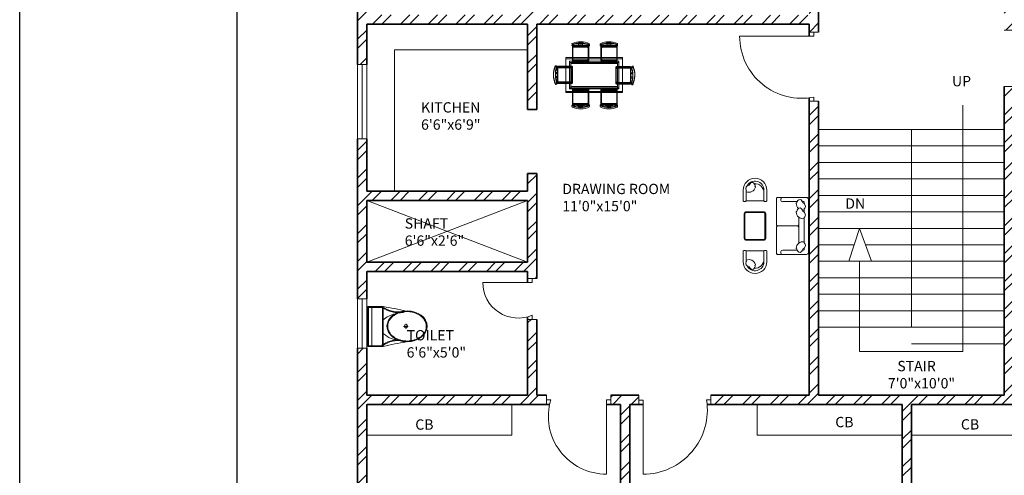
# Model space of a CAD drawing. Units: inches. Extents: x 2168 to 3056, y 1130 to 2629.
# Tile 2 of 42: x 2168 to 2645, y 1568 to 1789. Entities that reach past the tile are written whole.
import ezdxf

# ---------------------------------------------------------------- set-up
doc = ezdxf.new("R2010")
doc.units = ezdxf.units.IN
for name, color, linetype, lineweight in [('A-ANNO-DIMS', 2, 'Continuous', 18), ('A-ANNO-TEXT', 7, 'Continuous', 18), ('A-ANNO-TTLB', 7, 'Continuous', 25), ('A-AREA-IDEN', 7, 'Continuous', 18), ('A-DOOR', 21, 'Continuous', 18), ('A-FLOR-CASE', 71, 'Continuous', 18), ('A-FLOR-FIXT', 9, 'Continuous', 18), ('A-FLOR-OTLN', 7, 'Continuous', 18), ('A-FLOR-STRS', 71, 'Continuous', 18), ('A-FURN', 8, 'Continuous', 13), ('A-GLAZ', 201, 'Continuous', 18), ('A-WALL', 7, 'Continuous', 35)]:
    doc.layers.add(name, color=color, linetype=linetype, lineweight=lineweight)
doc.layers.add('A-WALL-PATT', color=143, linetype='Continuous', lineweight=13, true_color=0x7aafdf)
doc.styles.get("Standard").update_dxf_attribs({"font": 'arial.ttf'})
doc.dimstyles.get("Standard").update_dxf_attribs({"dimtxt": 0.18, "dimasz": 0.18, "dimexe": 0.18, "dimexo": 0.0625, "dimgap": 0.09, "dimtad": 0, "dimtih": 1, "dimtoh": 1, "dimdec": 4, "dimzin": 0, "dimdsep": 46, "dimtxsty": 'Standard', "dimcen": 0.09, "dimadec": 0, "dimazin": 0, "dimtfac": 1, "dimtdec": 4, "dimtofl": 0, "dimtmove": 0, "dimatfit": 3, "dimfxl": 1, "dimtolj": 1, "dimtzin": 0, "dimarcsym": 0})

# ---------------------------------------------------------------- blocks, each defined once
blk = doc.blocks.new('A$C31115884')
for p, q in [((258, 466), (258, 523)), ((283, 498), (223, 498)), ((0, 200), (0, 0)), ((520, 200), (0, 200)), ((10, 190), (10, 10)), ((510, 190), (10, 190)), ((510, 10), (510, 190)), ((520, 0), (520, 200)), ((510, 54), (0, 54)), ((10, 10), (510, 10)), ((0, 0), (520, 0))]:
    blk.add_line(p, q)
blk.add_circle((256, 496), 23.6)
for centre, radius, start, end in [((2778, -205), 2807, 165.4549, 171.7133), ((-295, 403), 365, 324.2091, 9.3499), ((-295, 403), 375, 324.2091, 9.3499), ((139, 406), 293, 315.8436, 2.6563), ((806, 403), 375, 179.2036, 215.7909), ((806, 403), 365, 170.6501, 215.7909), ((3237, 905), 2807, 188.2867, 194.5451), ((384, 406), 293, 190.2774, 224.1564)]:
    blk.add_arc(centre, radius, start, end)
blk.add_ellipse((256, 510), major_axis=(0, -261), ratio=0.772727)
blk.add_open_spline([(256, 259), (263, 259), (270, 260), (288, 262), (299, 265), (320, 273), (330, 278), (350, 291), (360, 299), (378, 316), (386, 326), (402, 347), (409, 358), (421, 383), (427, 395), (436, 422), (440, 436), (445, 465), (447, 480), (448, 509), (448, 524), (445, 553), (443, 568), (436, 596), (432, 610), (422, 636), (416, 649), (402, 672), (395, 683), (379, 703), (370, 712), (351, 728), (341, 735), (321, 746), (310, 751), (289, 757), (278, 759), (256, 761), (245, 761), (223, 757), (212, 754), (191, 746), (181, 741), (161, 728), (151, 720), (133, 703), (125, 693), (110, 672), (103, 660), (90, 636), (85, 623), (76, 596), (72, 582), (67, 553), (66, 538), (64, 509), (65, 494), (68, 465), (70, 450), (77, 422), (81, 408), (91, 382), (97, 370), (111, 346), (118, 335), (135, 316), (144, 307), (162, 291), (172, 284), (193, 273), (203, 269), (225, 262), (236, 260), (250, 259), (253, 259), (256, 259)], degree=3, knots=[0, 0, 0, 0, 0.110105, 0.110105, 0.285049, 0.285049, 0.459994, 0.459994, 0.634938, 0.634938, 0.809882, 0.809882, 0.984827, 0.984827, 1.159771, 1.159771, 1.334715, 1.334715, 1.50966, 1.50966, 1.684604, 1.684604, 1.859549, 1.859549, 2.034493, 2.034493, 2.209437, 2.209437, 2.384382, 2.384382, 2.559326, 2.559326, 2.73427, 2.73427, 2.909215, 2.909215, 3.084159, 3.084159, 3.259103, 3.259103, 3.434048, 3.434048, 3.608992, 3.608992, 3.783936, 3.783936, 3.958881, 3.958881, 4.133825, 4.133825, 4.30877, 4.30877, 4.483714, 4.483714, 4.658658, 4.658658, 4.833603, 4.833603, 5.008547, 5.008547, 5.183491, 5.183491, 5.358436, 5.358436, 5.53338, 5.53338, 5.708324, 5.708324, 5.883269, 5.883269, 6.058213, 6.058213, 6.233158, 6.233158, 6.283185, 6.283185, 6.283185, 6.283185])
blk = doc.blocks.new('A$C1352')
at = {"color": 0}
for points in [[(0.003, 0.053), (0.003, 0.553, -0.414214), (0.053, 0.603), (0.753, 0.603, -0.414214), (0.803, 0.553), (0.803, 0.053, -0.414214), (0.753, 0.003), (0.053, 0.003, -0.414214)], [(0.023, 0.053), (0.023, 0.553, -0.414214), (0.053, 0.583), (0.753, 0.583, -0.414214), (0.783, 0.553), (0.783, 0.053, -0.414214), (0.753, 0.023), (0.053, 0.023, -0.414214)]]:
    blk.add_lwpolyline(points, format="xyb", close=True, dxfattribs=at)
blk = doc.blocks.new('CHAIR-LOUNGE')
blk.add_line((10.04, 5.71), (10.04, 10.98))
at = {"ltscale": 0.03}
blk.add_lwpolyline([(10.04, 10.98, -0.369229), (11.42, 10.98), (11.42, 5.7, -1), (0, 5.72), (0, 10.99, -0.369229), (1.39, 10.99)], format="xyb", close=True, dxfattribs=at)
blk.add_lwpolyline([(9.55, 3.71, -0.785087), (1.38, 5.71), (1.39, 10.99)], format="xyb")
for centre, radius, start, end in [((5.71, 6.93), 4.33, 179.9461, 273.658), ((8.67, 3.43), 3.35, 67.0143, 164.2857), ((8.41, 5.02), 1.73, 272.9922, 34.1401), ((5.71, 5.71), 4.33, 358.8536, 359.9461), ((5.63, 4.23), 0.207, 150.6238, 293.7423), ((7.44, 3.63), 1.78, 166.6403, 249.4695), ((6.65, 3.91), 1.95, 274.9999, 341.3534)]:
    blk.add_arc(centre, radius, start, end)
blk = doc.blocks.new('TABLE-DINING')
for points in [[(0, 17.02), (27.45, 17.02), (27.45, 0.55), (0, 0.55)], [(0, 17.02), (27.45, 17.02), (27.45, 0.55), (0, 0.55)], [(0, 16.47), (27.45, 16.47), (27.45, 0), (0, 0)], [(0, 16.47), (27.45, 16.47), (27.45, 0), (0, 0)], [(1.83, 15.19), (25.62, 15.19), (25.62, 2.38), (1.83, 2.38)], [(1.83, 15.19), (25.62, 15.19), (25.62, 2.38), (1.83, 2.38)], [(1.83, 14.64), (25.62, 14.64), (25.62, 1.83), (1.83, 1.83)], [(1.83, 14.64), (25.62, 14.64), (25.62, 1.83), (1.83, 1.83)], [(2.38, 14.64), (25.07, 14.64), (25.07, 2.93), (2.38, 2.93)], [(2.38, 14.64), (25.07, 14.64), (25.07, 2.93), (2.38, 2.93)], [(2.38, 14.09), (25.07, 14.09), (25.07, 2.38), (2.38, 2.38)], [(2.38, 14.09), (25.07, 14.09), (25.07, 2.38), (2.38, 2.38)]]:
    blk.add_lwpolyline(points, close=True)
blk = doc.blocks.new('CUPBOARD-BEDROOM')
blk.add_lwpolyline([(0, 14.89), (70.36, 14.89), (70.36, 0), (0, 0)], close=True)
blk = doc.blocks.new('CHAIR-DINING-SIDE')
for points in [[(7.85, 2.38, 0.414214), (8.33, 2.86), (8.33, 9.24, 0.414214), (7.85, 9.73), (0.91, 9.73, 0.414214), (0.42, 9.24), (0.42, 2.86, 0.414214), (0.91, 2.38), (7.85, 2.38)], [(7.85, 2.38, 0.414214), (8.33, 2.86), (8.33, 9.24, 0.414214), (7.85, 9.73), (0.91, 9.73, 0.414214), (0.42, 9.24), (0.42, 2.86, 0.414214), (0.91, 2.38), (7.85, 2.38)], [(7.85, 1.83, 0.414214), (8.33, 2.31), (8.33, 8.69, 0.414214), (7.85, 9.18), (0.91, 9.18, 0.414214), (0.42, 8.69), (0.42, 2.31, 0.414214), (0.91, 1.83), (7.85, 1.83)], [(7.85, 1.83, 0.414214), (8.33, 2.31), (8.33, 8.69, 0.414214), (7.85, 9.18), (0.91, 9.18, 0.414214), (0.42, 8.69), (0.42, 2.31, 0.414214), (0.91, 1.83), (7.85, 1.83)], [(8.06, 2.08, -0.175809), (0.59, 2.13, 0.578392), (0.02, 1.51, 0.214524), (8.46, 1.4, 0.552014), (8.06, 2.08, -0.065079)], [(8.06, 2.08, -0.175809), (0.59, 2.13, 0.578392), (0.02, 1.51, 0.214524), (8.46, 1.4, 0.552014), (8.06, 2.08, -0.065079)], [(8.06, 1.53, -0.175809), (0.59, 1.58, 0.578392), (0.02, 0.96, 0.214524), (8.46, 0.85, 0.552014), (8.06, 1.53, -0.065079)], [(8.06, 1.53, -0.175809), (0.59, 1.58, 0.578392), (0.02, 0.96, 0.214524), (8.46, 0.85, 0.552014), (8.06, 1.53, -0.065079)], [(3.34, 2.38), (3.34, 1.5, -0.064759)], [(3.34, 2.38), (3.34, 1.5, -0.064759)], [(3.34, 1.83), (3.34, 0.95, -0.064759)], [(3.34, 1.83), (3.34, 0.95, -0.064759)]]:
    blk.add_lwpolyline(points, format="xyb")
for points in [[(7.84, 2.6), (1.13, 2.6, -0.414214), (0.64, 3.08), (0.64, 9.02, -0.414214), (1.13, 9.51), (7.84, 9.51, -0.512069), (8.11, 9.02), (8.11, 3.08, -0.512069)], [(7.84, 2.6), (1.13, 2.6, -0.414214), (0.64, 3.08), (0.64, 9.02, -0.414214), (1.13, 9.51), (7.84, 9.51, -0.512069), (8.11, 9.02), (8.11, 3.08, -0.512069)], [(7.84, 2.05), (1.13, 2.05, -0.414214), (0.64, 2.53), (0.64, 8.48, -0.414214), (1.13, 8.96), (7.84, 8.96, -0.512069), (8.11, 8.48), (8.11, 2.53, -0.512069)], [(7.84, 2.05), (1.13, 2.05, -0.414214), (0.64, 2.53), (0.64, 8.48, -0.414214), (1.13, 8.96), (7.84, 8.96, -0.512069), (8.11, 8.48), (8.11, 2.53, -0.512069)]]:
    blk.add_lwpolyline(points, format="xyb", close=True)
for points in [[(5.29, 1.48), (5.29, 2.38)], [(5.29, 1.48), (5.29, 2.38)], [(5.29, 0.93), (5.29, 1.83)], [(5.29, 0.93), (5.29, 1.83)]]:
    blk.add_lwpolyline(points)
blk = doc.blocks.new('CHAIR-DINING-END')
for points in [[(1.58, 1.14, -0.578392), (0.96, 0.57, -0.214524), (0.85, 9.01, -0.552014), (1.53, 8.61, 0.175809), (1.58, 1.14)], [(1.58, 1.14, -0.578392), (0.96, 0.57, -0.214524), (0.85, 9.01, -0.552014), (1.53, 8.61, 0.175809), (1.58, 1.14)], [(1.58, 0.59, -0.578392), (0.96, 0.02, -0.214524), (0.85, 8.46, -0.552014), (1.53, 8.06, 0.175809), (1.58, 0.59)], [(1.58, 0.59, -0.578392), (0.96, 0.02, -0.214524), (0.85, 8.46, -0.552014), (1.53, 8.06, 0.175809), (1.58, 0.59)], [(1.83, 8.39, -0.414214), (2.31, 8.88), (8.69, 8.88, -0.414214), (9.18, 8.39), (9.18, 1.45, -0.414214), (8.69, 0.97), (2.31, 0.97, -0.414214), (1.83, 1.45), (1.83, 8.39)], [(1.83, 8.39, -0.414214), (2.31, 8.88), (8.69, 8.88, -0.414214), (9.18, 8.39), (9.18, 1.45, -0.414214), (8.69, 0.97), (2.31, 0.97, -0.414214), (1.83, 1.45), (1.83, 8.39)], [(1.83, 7.85, -0.414214), (2.31, 8.33), (8.69, 8.33, -0.414214), (9.18, 7.85), (9.18, 0.91, -0.414214), (8.69, 0.42), (2.31, 0.42, -0.414214), (1.83, 0.91), (1.83, 7.85)], [(1.83, 7.85, -0.414214), (2.31, 8.33), (8.69, 8.33, -0.414214), (9.18, 7.85), (9.18, 0.91, -0.414214), (8.69, 0.42), (2.31, 0.42, -0.414214), (1.83, 0.91), (1.83, 7.85)], [(1.83, 3.89), (0.95, 3.89, 0.064759)], [(1.83, 3.89), (0.95, 3.89, 0.064759)], [(1.83, 3.34), (0.95, 3.34, 0.064759)], [(1.83, 3.34), (0.95, 3.34, 0.064759)]]:
    blk.add_lwpolyline(points, format="xyb")
for points in [[(0.93, 5.84), (1.83, 5.84)], [(0.93, 5.83), (1.83, 5.83)], [(0.93, 5.29), (1.83, 5.29)], [(0.93, 5.29), (1.83, 5.29)]]:
    blk.add_lwpolyline(points)
for points in [[(2.05, 8.39), (2.05, 1.67, 0.414214), (2.53, 1.19), (8.48, 1.19, 0.414214), (8.96, 1.67), (8.96, 8.39, 0.512069), (8.48, 8.66), (2.53, 8.66, 0.512069)], [(2.05, 8.39), (2.05, 1.67, 0.414214), (2.53, 1.19), (8.48, 1.19, 0.414214), (8.96, 1.67), (8.96, 8.39, 0.512069), (8.48, 8.66), (2.53, 8.66, 0.512069)], [(2.05, 7.84), (2.05, 1.12, 0.414214), (2.53, 0.64), (8.48, 0.64, 0.414214), (8.96, 1.12), (8.96, 7.84, 0.512069), (8.48, 8.11), (2.53, 8.11, 0.512069)], [(2.05, 7.84), (2.05, 1.12, 0.414214), (2.53, 0.64), (8.48, 0.64, 0.414214), (8.96, 1.12), (8.96, 7.84, 0.512069), (8.48, 8.11), (2.53, 8.11, 0.512069)]]:
    blk.add_lwpolyline(points, format="xyb", close=True)
blk = doc.blocks.new('WIN-24-OPPOSED-JAMBS')
for p, q in [((0, 4.5), (0, 0)), ((0, 4.5), (24, 4.5)), ((0, 0), (0, 2.25)), ((0, 2.25), (24, 2.25)), ((24, 2.25), (24, 4.5)), ((24, 4.5), (24, 0)), ((0, 0), (24, 0))]:
    blk.add_line(p, q)
blk = doc.blocks.new('WIN-36')
for p, q in [((2.25, 36), (0, 36)), ((0, 36), (4.5, 36)), ((0, 36), (0, 0)), ((2.25, 0), (2.25, 36)), ((4.5, 36), (4.5, 0)), ((0, 0), (4.5, 0)), ((4.5, 0), (2.25, 0))]:
    blk.add_line(p, q)
blk = doc.blocks.new('*D41')
at = {"layer": 'A-ANNO-DIMS', "color": 0, "lineweight": -2, "transparency": 16777216}
for p, q in [((2331.73, 2478.39), (2273.32, 2478.39)), ((2273.5, 2478.21), (2273.5, 1928.07)), ((2273.5, 1377.57), (2273.5, 1927.71)), ((2331.73, 1377.39), (2273.32, 1377.39))]:
    blk.add_line(p, q, dxfattribs=at)
at = {"layer": 'A-ANNO-DIMS', "color": 0, "transparency": 16777216}
for points in [[(2273.47, 2478.21), (2273.53, 2478.21), (2273.5, 2478.39)], [(2273.47, 1377.57), (2273.53, 1377.57), (2273.5, 1377.39)]]:
    blk.add_solid(points, dxfattribs=at)
at = {"layer": 'Defpoints', "color": 0, "transparency": 16777216}
for p in [(2273.5, 2478.39), (2331.8, 2478.39), (2331.8, 1377.39)]:
    blk.add_point(p, dxfattribs=at)
at = {"layer": 'A-ANNO-DIMS', "color": 0, "transparency": 16777216, "insert": (2273.5, 1927.89), "char_height": 0.18, "attachment_point": 5}
blk.add_mtext('\\A1;1101', dxfattribs=at)

msp = doc.modelspace()

# ---------------------------------------------------------------- hatches: boundary and pattern name
at = {"layer": 'A-WALL-PATT'}
h = msp.add_hatch(dxfattribs=at)
h.set_pattern_fill('ANSI32', color=256)
h.paths.add_polyline_path([(2463.8, 2409.39), (2467.39, 2409.39), (2467.39, 2413.89), (2454.77, 2413.89), (2454.77, 2411.64), (2454.77, 2409.39), (2459.3, 2409.39), (2459.3, 2265.39), (2455.64, 2265.39), (2455.64, 2260.89), (2467.35, 2260.89), (2467.35, 2263.14), (2467.35, 2265.39), (2463.8, 2265.39)])
h.paths.add_polyline_path([(2431.6, 2413.89), (2409.65, 2413.89), (2409.65, 2409.39), (2431.6, 2409.39), (2431.6, 2411.64)])
h.paths.add_polyline_path([(2349.65, 2413.89), (2331.8, 2413.89), (2331.8, 2362.67), (2336.3, 2362.67), (2336.3, 2409.39), (2349.65, 2409.39), (2349.65, 2411.64)])
h.paths.add_polyline_path([(2634.15, 2411.64), (2634.15, 2413.89), (2562.29, 2413.89), (2562.29, 2409.39), (2595.8, 2409.39), (2595.8, 2280.31), (2595.83, 2280.31), (2595.83, 2265.39), (2499.91, 2265.39), (2499.91, 2260.89), (2550.8, 2260.89), (2550.8, 2117.31), (2555.3, 2117.31), (2555.3, 2168.08), (2571.93, 2168.08), (2571.93, 2176.89), (2559.8, 2176.89), (2559.8, 2256.39), (2640.8, 2256.39), (2640.8, 2176.89), (2626.43, 2176.89), (2626.43, 2168.08), (2645.3, 2168.08), (2645.3, 2116.64), (2649.8, 2116.64), (2649.8, 2260.89), (2691.25, 2260.89), (2691.25, 2263.14), (2691.25, 2265.39), (2670.65, 2265.39), (2670.65, 2265.36), (2600.3, 2265.36), (2600.3, 2280.26), (2600.3, 2409.39), (2634.15, 2409.39)])
h.paths.add_polyline_path([(2600.3, 2473.89), (2612.84, 2473.89), (2612.84, 2478.39), (2572.64, 2478.39), (2572.64, 2473.89), (2595.8, 2473.89), (2595.8, 2413.89), (2600.3, 2413.89)])
h.paths.add_polyline_path([(2535.8, 2473.89), (2548.64, 2473.89), (2548.64, 2478.39), (2531.4, 2478.39), (2531.4, 2413.89), (2521.6, 2413.89), (2521.6, 2409.39), (2539.24, 2409.39), (2539.24, 2411.64), (2539.24, 2413.89), (2535.8, 2413.89)])
h.paths.add_polyline_path([(2664.8, 2478.39), (2636.84, 2478.39), (2636.84, 2473.89), (2660.3, 2473.89), (2660.3, 2413.89), (2656.17, 2413.89), (2656.17, 2409.39), (2671.68, 2409.39), (2671.68, 2411.64), (2671.68, 2413.89), (2664.8, 2413.89)])
h.paths.add_polyline_path([(2705.94, 2413.89), (2695.68, 2413.89), (2695.68, 2409.39), (2705.94, 2409.39)])
h.paths.add_polyline_path([(2741.35, 2413.89), (2728.73, 2413.89), (2728.73, 2411.64), (2728.73, 2409.39), (2732.3, 2409.39), (2732.3, 2265.39), (2725.73, 2265.39), (2725.73, 2260.89), (2740.92, 2260.89), (2740.92, 2263.14), (2740.92, 2265.39), (2736.8, 2265.39), (2736.8, 2409.39), (2741.35, 2409.39)])
h.paths.add_polyline_path([(2785.65, 2413.89), (2764.55, 2413.89), (2764.49, 2409.39), (2785.65, 2409.39), (2785.65, 2411.64)])
h.paths.add_polyline_path([(2864.3, 2413.89), (2845.65, 2413.89), (2845.65, 2409.39), (2859.8, 2409.39), (2859.8, 2368.43), (2864.3, 2368.43)])
h.paths.add_polyline_path([(2864.3, 2308.43), (2862.05, 2308.43), (2859.8, 2308.43), (2859.8, 2265.39), (2774.48, 2265.39), (2774.48, 2263.14), (2774.48, 2260.89), (2781.8, 2260.89), (2781.8, 2226.65), (2786.3, 2226.65), (2786.3, 2260.89), (2859.8, 2260.89), (2859.8, 2241.35), (2864.3, 2241.35)])
h.paths.add_polyline_path([(2864.3, 2217.35), (2862.05, 2217.35), (2859.8, 2217.35), (2859.8, 2200.89), (2786.3, 2200.89), (2786.3, 2205.93), (2784.05, 2205.93), (2781.8, 2205.93), (2781.8, 2150.97), (2786.3, 2150.97), (2786.3, 2161.89), (2859.8, 2161.89), (2859.8, 2144.42), (2864.3, 2144.42)])
h.paths.add_polyline_path([(2859.8, 2196.39), (2859.8, 2166.39), (2786.3, 2166.39), (2786.3, 2196.39)], flags=16)
h.paths.add_polyline_path([(2864.3, 2108.42), (2862.05, 2108.42), (2859.8, 2108.42), (2859.8, 2080.89), (2786.3, 2080.89), (2786.3, 2111.99), (2781.8, 2111.99), (2781.8, 2080.89), (2649.8, 2080.89), (2649.8, 2086.04), (2647.55, 2086.04), (2645.3, 2086.04), (2645.3, 2071.74), (2649.8, 2071.74), (2649.8, 2076.39), (2781.8, 2076.39), (2781.8, 2041.79), (2786.3, 2041.79), (2786.3, 2076.39), (2859.8, 2076.39), (2859.8, 2058.58), (2864.3, 2058.58)])
h.paths.add_polyline_path([(2864.3, 2022.58), (2859.8, 2022.58), (2859.8, 1992.39), (2786.3, 1992.39), (2786.3, 1999.57), (2781.8, 1999.57), (2781.8, 1848.09), (2784.05, 1848.09), (2786.3, 1848.09), (2786.3, 1851.39), (2859.8, 1851.39), (2859.8, 1838.26), (2864.3, 1838.26)], flags=17)
h.paths.add_polyline_path([(2859.8, 1987.89), (2859.8, 1855.89), (2786.3, 1855.89), (2786.3, 1987.89)], flags=16)
h.paths.add_polyline_path([(2823.05, 1987.89), (2841.42, 1921.89), (2823.05, 1855.89)], flags=0)
h.paths.add_polyline_path([(2864.3, 1814.26), (2859.8, 1814.26), (2859.8, 1791.39), (2786.3, 1791.39), (2786.3, 1825.66), (2784.05, 1825.66), (2781.8, 1825.66), (2781.8, 1791.39), (2720.15, 1791.39), (2720.15, 1791.27), (2649.8, 1791.27), (2649.8, 1806.16), (2649.8, 2038.98), (2647.55, 2038.98), (2645.3, 2038.98), (2645.3, 1783.93), (2649.8, 1783.93), (2649.8, 1786.89), (2781.8, 1786.89), (2781.8, 1746.79), (2786.3, 1746.79), (2786.3, 1786.89), (2859.8, 1786.89), (2859.8, 1770.08), (2864.3, 1770.08)])
h.paths.add_polyline_path([(2864.3, 1734.08), (2862.05, 1734.08), (2859.8, 1734.08), (2859.8, 1705.89), (2786.3, 1705.89), (2786.3, 1714.17), (2781.8, 1714.17), (2781.8, 1660.53), (2786.3, 1660.53), (2786.3, 1666.89), (2859.8, 1666.89), (2859.8, 1648.34), (2864.3, 1648.34)])
h.paths.add_polyline_path([(2786.3, 1701.39), (2859.8, 1701.39), (2859.8, 1671.39), (2786.3, 1671.39)], flags=16)
h.paths.add_polyline_path([(2649.8, 1756.58), (2647.55, 1756.58), (2645.3, 1756.58), (2645.3, 1606.89), (2555.3, 1606.89), (2555.3, 1749.51), (2553.05, 1749.51), (2550.8, 1749.51), (2550.8, 1606.89), (2503.01, 1606.89), (2503.01, 1604.64), (2503.01, 1602.39), (2595.8, 1602.39), (2595.85, 1602.39), (2595.85, 1587.5), (2595.8, 1458.39), (2561.5, 1458.39), (2561.5, 1456.14), (2561.5, 1453.89), (2595.8, 1453.89), (2595.8, 1381.89), (2573.44, 1381.89), (2573.44, 1377.39), (2613.01, 1377.39), (2613.01, 1379.64), (2613.01, 1381.89), (2600.3, 1381.89), (2600.3, 1453.89), (2634.33, 1453.89), (2634.33, 1458.39), (2600.3, 1458.39), (2600.3, 1602.39), (2670.65, 1602.39), (2694.09, 1602.39), (2694.09, 1606.89), (2649.8, 1606.89)])
h.paths.add_polyline_path([(2736.8, 1602.39), (2741.56, 1602.39), (2741.56, 1606.89), (2726.2, 1606.89), (2726.2, 1604.64), (2726.2, 1602.39), (2732.3, 1602.39), (2732.3, 1458.39), (2727.9, 1458.39), (2727.9, 1453.89), (2740.82, 1453.89), (2740.82, 1456.14), (2740.82, 1458.39), (2736.8, 1458.39)])
h.paths.add_polyline_path([(2859.8, 1606.89), (2786.3, 1606.89), (2786.3, 1637.33), (2784.05, 1637.33), (2781.8, 1637.33), (2781.8, 1606.89), (2775.61, 1606.89), (2775.61, 1602.39), (2859.8, 1602.39)])
h.paths.add_polyline_path([(2864.3, 1624.34), (2862.05, 1624.34), (2859.8, 1624.34), (2859.8, 1570.39), (2864.3, 1570.39)])
h.paths.add_polyline_path([(2864.3, 1510.39), (2862.05, 1510.39), (2859.8, 1510.39), (2859.8, 1458.39), (2846.73, 1458.39), (2846.73, 1456.14), (2846.73, 1453.89), (2864.3, 1453.89)])
h.paths.add_polyline_path([(2786.73, 1458.39), (2765.44, 1458.39), (2765.44, 1453.89), (2786.73, 1453.89)])
h.paths.add_polyline_path([(2706, 1458.39), (2695.36, 1458.39), (2695.36, 1453.89), (2706, 1453.89), (2706, 1456.14)])
h.paths.add_polyline_path([(2671.36, 1456.14), (2671.36, 1458.39), (2655.99, 1458.39), (2655.99, 1456.14), (2655.99, 1453.89), (2660.3, 1453.89), (2660.3, 1381.89), (2637.01, 1381.89), (2637.01, 1377.39), (2664.8, 1377.39), (2664.8, 1453.89), (2671.36, 1453.89)], flags=17)
h.paths.add_polyline_path([(2539.83, 1458.39), (2520.24, 1458.39), (2520.24, 1453.89), (2531.3, 1453.89), (2531.3, 1377.39), (2546.45, 1377.39), (2546.45, 1379.64), (2546.45, 1381.89), (2535.8, 1381.89), (2535.8, 1453.89), (2539.83, 1453.89)], flags=17)
h.paths.add_polyline_path([(2496.24, 1458.39), (2489.13, 1458.39), (2489.13, 1453.89), (2496.24, 1453.89), (2496.24, 1456.14)])
h.paths.add_polyline_path([(2467.43, 1456.14), (2467.43, 1458.39), (2463.8, 1458.39), (2463.8, 1602.39), (2468.24, 1602.39), (2468.24, 1605.7), (2468.24, 1606.89), (2454.6, 1606.89), (2454.6, 1602.39), (2459.3, 1602.39), (2459.3, 1458.39), (2454.24, 1458.39), (2454.24, 1453.89), (2467.43, 1453.89)])
h.paths.add_polyline_path([(2431.6, 1456.14), (2431.6, 1458.39), (2411.39, 1458.39), (2411.39, 1453.89), (2431.6, 1453.89)])
h.paths.add_polyline_path([(2351.39, 1458.39), (2336.3, 1458.39), (2336.3, 1490.69), (2334.05, 1490.69), (2331.8, 1490.69), (2331.8, 1453.89), (2351.39, 1453.89), (2351.39, 1456.14)])
h.paths.add_polyline_path([(2336.3, 1629.7), (2331.8, 1629.7), (2331.8, 1552.32), (2336.3, 1552.32), (2336.3, 1602.39), (2406.65, 1602.39), (2423.47, 1602.39), (2423.47, 1606.89), (2418.8, 1606.89), (2418.8, 1643.68), (2416.55, 1643.68), (2414.3, 1643.68), (2414.3, 1606.89), (2336.3, 1606.89)])
h.paths.add_polyline_path([(2418.8, 1714.38), (2414.3, 1714.38), (2414.3, 1705.89), (2336.3, 1705.89), (2336.3, 1731.32), (2334.05, 1731.32), (2331.8, 1731.32), (2331.8, 1653.7), (2334.05, 1653.7), (2336.3, 1653.7), (2336.3, 1666.89), (2414.3, 1666.89), (2414.3, 1663.59), (2418.8, 1663.59)])
h.paths.add_polyline_path([(2336.3, 1701.39), (2414.3, 1701.39), (2414.3, 1671.39), (2336.3, 1671.39)], flags=16)
h.paths.add_polyline_path([(2555.3, 2040.06), (2550.8, 2040.06), (2550.8, 1791.39), (2550.56, 1791.2), (2480.2, 1791.2), (2418.8, 1791.39), (2418.8, 1825.45), (2416.55, 1825.45), (2414.3, 1825.45), (2414.3, 1791.39), (2336.3, 1791.39), (2336.3, 1806.41), (2331.8, 1806.41), (2331.8, 1767.32), (2336.3, 1767.32), (2336.3, 1786.89), (2414.3, 1786.89), (2414.3, 1745.46), (2418.8, 1745.46), (2418.8, 1786.89), (2550.8, 1786.89), (2550.8, 1783.01), (2555.3, 1783.01)])
h.paths.add_polyline_path([(2418.8, 1923.39), (2423.21, 1923.39), (2423.21, 1925.64), (2423.21, 1927.89), (2418.8, 1927.89), (2418.8, 2000.05), (2414.3, 2000.05), (2414.3, 1992.39), (2336.3, 1992.39), (2336.3, 1987.89), (2414.3, 1987.89), (2414.3, 1855.89), (2336.3, 1855.89), (2336.3, 1851.39), (2414.3, 1851.39), (2414.3, 1846.76), (2418.8, 1846.76)], flags=17)
h.paths.add_polyline_path([(2336.3, 2019.29), (2334.05, 2019.29), (2331.8, 2019.29), (2331.8, 1830.41), (2336.3, 1830.41)], flags=17)
h.paths.add_polyline_path([(2550.8, 1927.89), (2453.54, 1927.89), (2453.54, 1925.64), (2453.54, 1923.39), (2550.8, 1923.39)], flags=17)
h.paths.add_polyline_path([(2744.99, 1927.89), (2649.8, 1927.89), (2649.8, 1923.39), (2744.99, 1923.39), (2744.99, 1925.64)], flags=17)
h.paths.add_polyline_path([(2555.3, 2086.46), (2553.05, 2086.46), (2550.8, 2086.46), (2550.8, 2080.89), (2418.8, 2080.89), (2336.3, 2080.89), (2336.3, 2115.4), (2334.05, 2115.4), (2331.8, 2115.4), (2331.8, 2055.29), (2336.3, 2055.29), (2336.3, 2076.39), (2550.8, 2076.39), (2550.8, 2071.54), (2555.3, 2071.54)])
h.paths.add_polyline_path([(2418.8, 2121.39), (2414.3, 2121.39), (2414.3, 2080.89), (2418.8, 2080.89)])
h.paths.add_polyline_path([(2418.8, 2076.39), (2414.3, 2076.39), (2414.3, 2035.12), (2418.8, 2035.12)])
h.paths.add_polyline_path([(2422.87, 2263.14), (2422.87, 2265.39), (2406.65, 2265.39), (2406.65, 2265.36), (2336.3, 2265.36), (2336.3, 2280.25), (2336.3, 2302.67), (2334.05, 2302.67), (2331.8, 2302.67), (2331.8, 2246.85), (2336.3, 2246.85), (2336.3, 2260.89), (2414.3, 2260.89), (2414.3, 2224), (2418.8, 2224), (2418.8, 2260.89), (2422.87, 2260.89)])
h.paths.add_polyline_path([(2418.8, 2204.78), (2416.55, 2204.78), (2414.3, 2204.78), (2414.3, 2200.89), (2336.3, 2200.89), (2336.3, 2220.85), (2331.8, 2220.85), (2331.8, 2151.4), (2336.3, 2151.4), (2336.3, 2161.89), (2414.3, 2161.89), (2414.3, 2153.73), (2418.8, 2153.73)])
h.paths.add_polyline_path([(2414.3, 2196.39), (2414.3, 2166.39), (2336.3, 2166.39), (2336.3, 2196.39)], flags=16)
h.paths.add_polyline_path([(2375.3, 2181.39), (2336.3, 2166.39), (2336.3, 2196.39)], flags=0)
h.paths.add_polyline_path([(2809.6, 2172.34), (2838.8, 2172.34), (2838.8, 2191), (2809.6, 2191)], flags=8)
h.paths.add_polyline_path([(2849.75, 1919.59), (2849.75, 1952.67), (2831.09, 1952.67), (2831.09, 1919.59)], flags=8)
h.paths.add_polyline_path([(2808.87, 1901.97), (2808.87, 1937.85), (2790.15, 1937.85), (2790.15, 1901.97)], flags=8)
h.paths.add_polyline_path([(2806.28, 1671.9), (2835.49, 1671.9), (2835.49, 1690.55), (2806.28, 1690.55)], flags=8)
h.paths.add_polyline_path([(2353.19, 1676.55), (2382.39, 1676.55), (2382.39, 1695.21), (2353.19, 1695.21)], flags=8)
h.paths.add_polyline_path([(2360.08, 1832.31), (2389.24, 1832.31), (2389.24, 1850.97), (2360.08, 1850.97)], flags=25)
h.paths.add_polyline_path([(2354.82, 2167.82), (2384.03, 2167.82), (2384.03, 2186.48), (2354.82, 2186.48)], flags=8)

# ---------------------------------------------------------------- linework, layer by layer
at = {"layer": 'A-ANNO-TTLB'}
msp.add_lwpolyline([(2168.16, 2629.19), (3055.63, 2629.19), (3055.63, 1130.19), (2168.16, 1130.19)], close=True, dxfattribs=at)
at = {"layer": 'A-DOOR'}
for p, q in [((2553.05, 1781.01), (2517.05, 1781.01)), ((2550.8, 1783.01), (2555.3, 1783.01)), ((2555.3, 1783.01), (2553.05, 1783.01)), ((2553.05, 1783.01), (2553.05, 1781.01)), ((2645.3, 1783.93), (2649.8, 1783.93)), ((2645.3, 1756.58), (2649.8, 1756.58)), ((2553.05, 1749.51), (2553.05, 1751.51)), ((2550.8, 1749.51), (2555.3, 1749.51)), ((2555.3, 1749.51), (2553.05, 1749.51)), ((2416.55, 1661.59), (2392.55, 1661.59)), ((2414.3, 1663.59), (2418.8, 1663.59)), ((2418.8, 1663.59), (2416.55, 1663.59)), ((2416.55, 1663.59), (2416.55, 1661.59)), ((2414.3, 1643.68), (2418.8, 1643.68)), ((2416.55, 1643.68), (2416.55, 1645.68)), ((2418.8, 1643.68), (2416.55, 1643.68)), ((2423.47, 1602.39), (2423.47, 1606.89)), ((2423.47, 1606.89), (2423.47, 1604.64)), ((2423.47, 1604.64), (2425.47, 1604.64)), ((2454.6, 1604.64), (2452.6, 1604.64)), ((2452.6, 1604.64), (2452.6, 1568.64)), ((2454.6, 1606.89), (2454.6, 1602.39)), ((2454.6, 1602.39), (2454.6, 1604.64)), ((2468.24, 1605.7), (2468.24, 1606.89)), ((2468.24, 1606.89), (2468.24, 1604.57)), ((2468.24, 1602.39), (2468.24, 1605.7)), ((2468.24, 1604.57), (2470.24, 1604.57)), ((2470.24, 1604.57), (2470.24, 1568.57)), ((2503.01, 1604.64), (2501.01, 1604.64)), ((2503.01, 1602.39), (2503.01, 1606.89)), ((2503.01, 1606.89), (2503.01, 1604.64))]:
    msp.add_line(p, q, dxfattribs=at)
for centre, radius, start, end in [((2547.13, 1781.01), 30.09, 180, 281.3384), ((2409.82, 1661.59), 17.27, 180, 292.9159), ((2452.44, 1596.74), 28.1, 163.6836, 270.3208), ((2470.24, 1599.73), 31.15, 270, 9.0691)]:
    msp.add_arc(centre, radius, start, end, dxfattribs=at)
at = {"layer": 'A-FLOR-CASE'}
for p, q in [((2414.3, 1774.45), (2349.78, 1774.45)), ((2349.78, 1774.45), (2349.78, 1705.89))]:
    msp.add_line(p, q, dxfattribs=at)
at = {"layer": 'A-FLOR-OTLN'}
for p, q in [((2336.3, 1671.39), (2414.3, 1701.39)), ((2336.3, 1701.39), (2414.3, 1671.39)), ((2414.3, 1701.39), (2414.3, 1701.39)), ((2336.3, 1671.39), (2336.3, 1671.39))]:
    msp.add_line(p, q, dxfattribs=at)
at = {"layer": 'A-FLOR-STRS'}
for p, q in [((2625.12, 1747.61), (2625.12, 1628.15)), ((2555.3, 1735.84), (2645.3, 1735.84)), ((2600.3, 1639.84), (2600.3, 1735.84)), ((2555.3, 1727.84), (2645.3, 1727.84)), ((2555.3, 1719.84), (2645.3, 1719.84)), ((2555.3, 1711.84), (2645.3, 1711.84)), ((2555.3, 1703.84), (2645.3, 1703.84)), ((2555.3, 1695.84), (2645.3, 1695.84)), ((2555.3, 1687.84), (2645.3, 1687.84)), ((2575.16, 1687.84), (2569.97, 1671.84)), ((2580.99, 1671.84), (2575.16, 1687.84)), ((2555.3, 1679.84), (2572.56, 1679.84)), ((2578.08, 1679.84), (2645.3, 1679.84)), ((2555.3, 1671.84), (2645.3, 1671.84)), ((2569.97, 1671.84), (2580.99, 1671.84)), ((2575.16, 1628.15), (2575.16, 1671.84)), ((2555.3, 1663.84), (2645.3, 1663.84)), ((2555.3, 1655.84), (2645.3, 1655.84)), ((2555.3, 1647.84), (2645.3, 1647.84)), ((2555.3, 1639.84), (2645.3, 1639.84)), ((2645.3, 1639.84), (2600.3, 1639.84)), ((2645.3, 1631.84), (2600.3, 1631.84)), ((2625.12, 1628.15), (2575.16, 1628.15))]:
    msp.add_line(p, q, dxfattribs=at)
at = {"layer": 'A-FURN'}
for p, q in [((2544.89, 1700.78), (2537.97, 1700.78)), ((2547.52, 1700.78), (2548, 1700.78)), ((2548.35, 1700.43), (2548.35, 1699.79)), ((2548.35, 1695.64), (2548.35, 1697.29)), ((2548.35, 1696.27), (2548.35, 1695.64)), ((2548.35, 1680.72), (2548.35, 1693.14)), ((2537.97, 1677.24), (2544.89, 1677.24)), ((2547.52, 1677.24), (2548, 1677.24)), ((2548.35, 1677.59), (2548.35, 1678.23))]:
    msp.add_line(p, q, dxfattribs=at)
for points in [[(2450.01, 1776.78, -0.578392), (2449.44, 1777.4, -0.214524), (2457.88, 1777.51, -0.552014), (2457.48, 1776.83, 0.175809), (2450.01, 1776.78)], [(2450.01, 1776.78, -0.578392), (2449.44, 1777.4, -0.214524), (2457.88, 1777.51, -0.552014), (2457.48, 1776.83, 0.175809), (2450.01, 1776.78)], [(2450.01, 1776.23, -0.578392), (2449.44, 1776.85, -0.214524), (2457.88, 1776.96, -0.552014), (2457.48, 1776.28, 0.175809), (2450.01, 1776.23)], [(2450.01, 1776.23, -0.578392), (2449.44, 1776.85, -0.214524), (2457.88, 1776.96, -0.552014), (2457.48, 1776.28, 0.175809), (2450.01, 1776.23)], [(2457.26, 1776.53, -0.414214), (2457.75, 1776.05), (2457.75, 1769.67, -0.414214), (2457.26, 1769.18), (2450.32, 1769.18, -0.414214), (2449.84, 1769.67), (2449.84, 1776.05, -0.414214), (2450.32, 1776.53), (2457.26, 1776.53)], [(2457.26, 1776.53, -0.414214), (2457.75, 1776.05), (2457.75, 1769.67, -0.414214), (2457.26, 1769.18), (2450.32, 1769.18, -0.414214), (2449.84, 1769.67), (2449.84, 1776.05, -0.414214), (2450.32, 1776.53), (2457.26, 1776.53)], [(2457.26, 1775.98, -0.414214), (2457.75, 1775.5), (2457.75, 1769.12, -0.414214), (2457.26, 1768.63), (2450.32, 1768.63, -0.414214), (2449.84, 1769.12), (2449.84, 1775.5, -0.414214), (2450.32, 1775.98), (2457.26, 1775.98)], [(2457.26, 1775.98, -0.414214), (2457.75, 1775.5), (2457.75, 1769.12, -0.414214), (2457.26, 1768.63), (2450.32, 1768.63, -0.414214), (2449.84, 1769.12), (2449.84, 1775.5, -0.414214), (2450.32, 1775.98), (2457.26, 1775.98)], [(2452.76, 1776.53), (2452.76, 1777.41, 0.064759)], [(2452.76, 1776.53), (2452.76, 1777.41, 0.064759)], [(2452.76, 1775.98), (2452.76, 1776.86, 0.064759)], [(2452.76, 1775.98), (2452.76, 1776.86, 0.064759)], [(2428.42, 1758.78, -0.578392), (2427.79, 1758.22, -0.214524), (2427.68, 1766.65, -0.552014), (2428.36, 1766.26, 0.175809), (2428.42, 1758.78)], [(2428.42, 1758.78, -0.578392), (2427.79, 1758.21, -0.214524), (2427.68, 1766.65, -0.552014), (2428.36, 1766.26, 0.175809), (2428.42, 1758.78)], [(2428.42, 1758.23, -0.578392), (2427.79, 1757.67, -0.214524), (2427.68, 1766.1, -0.552014), (2428.36, 1765.71, 0.175809), (2428.42, 1758.23)], [(2428.42, 1758.23, -0.578392), (2427.79, 1757.67, -0.214524), (2427.68, 1766.1, -0.552014), (2428.36, 1765.71, 0.175809), (2428.42, 1758.23)], [(2428.66, 1766.04, -0.414214), (2429.14, 1766.52), (2435.53, 1766.52, -0.414214), (2436.01, 1766.04), (2436.01, 1759.1, -0.414214), (2435.53, 1758.61), (2429.14, 1758.61, -0.414214), (2428.66, 1759.1), (2428.66, 1766.04)], [(2428.66, 1766.04, -0.414214), (2429.14, 1766.52), (2435.53, 1766.52, -0.414214), (2436.01, 1766.04), (2436.01, 1759.1, -0.414214), (2435.53, 1758.61), (2429.14, 1758.61, -0.414214), (2428.66, 1759.1), (2428.66, 1766.04)], [(2428.66, 1765.49, -0.414214), (2429.14, 1765.98), (2435.53, 1765.98, -0.414214), (2436.01, 1765.49), (2436.01, 1758.55, -0.414214), (2435.53, 1758.06), (2429.14, 1758.06, -0.414214), (2428.66, 1758.55), (2428.66, 1765.49)], [(2428.66, 1765.49, -0.414214), (2429.14, 1765.97), (2435.53, 1765.97, -0.414214), (2436.01, 1765.49), (2436.01, 1758.55, -0.414214), (2435.53, 1758.06), (2429.14, 1758.06, -0.414214), (2428.66, 1758.55), (2428.66, 1765.49)], [(2428.66, 1761.54), (2427.78, 1761.54, 0.064759)], [(2428.66, 1761.54), (2427.78, 1761.54, 0.064759)], [(2428.66, 1760.99), (2427.78, 1760.99, 0.064759)], [(2428.66, 1760.99), (2427.78, 1760.99, 0.064759)], [(2443.4, 1748.17), (2436.46, 1748.17, -0.414214), (2435.97, 1748.65), (2435.97, 1755.03, -0.414214), (2436.46, 1755.52), (2443.4, 1755.52, -0.414214), (2443.88, 1755.03), (2443.88, 1748.65, -0.414214), (2443.4, 1748.17)], [(2443.4, 1748.17), (2436.46, 1748.17, -0.414214), (2435.97, 1748.65), (2435.97, 1755.03, -0.414214), (2436.46, 1755.52), (2443.4, 1755.52, -0.414214), (2443.88, 1755.03), (2443.88, 1748.65, -0.414214), (2443.4, 1748.17)], [(2443.4, 1747.62), (2436.46, 1747.62, -0.414214), (2435.97, 1748.1), (2435.97, 1754.49, -0.414214), (2436.46, 1754.97), (2443.4, 1754.97, -0.414214), (2443.88, 1754.49), (2443.88, 1748.1, -0.414214), (2443.4, 1747.62)], [(2443.4, 1747.62), (2436.46, 1747.62, -0.414214), (2435.97, 1748.1), (2435.97, 1754.49, -0.414214), (2436.46, 1754.97), (2443.4, 1754.97, -0.414214), (2443.88, 1754.49), (2443.88, 1748.1, -0.414214), (2443.4, 1747.62)], [(2457.26, 1748.17, 0.414214), (2457.75, 1748.65), (2457.75, 1755.03, 0.414214), (2457.26, 1755.52), (2450.32, 1755.52, 0.414214), (2449.84, 1755.03), (2449.84, 1748.65, 0.414214), (2450.32, 1748.17), (2457.26, 1748.17)], [(2457.26, 1748.17, 0.414214), (2457.75, 1748.65), (2457.75, 1755.03, 0.414214), (2457.26, 1755.52), (2450.32, 1755.52, 0.414214), (2449.84, 1755.03), (2449.84, 1748.65, 0.414214), (2450.32, 1748.17), (2457.26, 1748.17)], [(2457.26, 1747.62, 0.414214), (2457.75, 1748.1), (2457.75, 1754.49, 0.414214), (2457.26, 1754.97), (2450.32, 1754.97, 0.414214), (2449.84, 1754.49), (2449.84, 1748.1, 0.414214), (2450.32, 1747.62), (2457.26, 1747.62)], [(2457.26, 1747.62, 0.414214), (2457.75, 1748.1), (2457.75, 1754.49, 0.414214), (2457.26, 1754.97), (2450.32, 1754.97, 0.414214), (2449.84, 1754.49), (2449.84, 1748.1, 0.414214), (2450.32, 1747.62), (2457.26, 1747.62)], [(2443.71, 1747.92, -0.578392), (2444.28, 1747.3, -0.214524), (2435.84, 1747.19, -0.552014), (2436.24, 1747.87, 0.175809), (2443.71, 1747.92)], [(2443.71, 1747.92, -0.578392), (2444.28, 1747.3, -0.214524), (2435.84, 1747.19, -0.552014), (2436.24, 1747.87, 0.175809), (2443.71, 1747.92)], [(2443.71, 1747.38, -0.578392), (2444.28, 1746.75, -0.214524), (2435.84, 1746.64, -0.552014), (2436.24, 1747.32, 0.175809), (2443.71, 1747.38)], [(2443.71, 1747.38, -0.578392), (2444.28, 1746.75, -0.214524), (2435.84, 1746.64, -0.552014), (2436.24, 1747.32, 0.175809), (2443.71, 1747.38)], [(2440.96, 1748.17), (2440.96, 1747.29, 0.064759)], [(2440.96, 1748.17), (2440.96, 1747.29, 0.064759)], [(2440.96, 1747.62), (2440.96, 1746.74, 0.064759)], [(2440.96, 1747.62), (2440.96, 1746.74, 0.064759)], [(2457.48, 1747.87, -0.175809), (2450.01, 1747.92, 0.578392), (2449.44, 1747.3, 0.214524), (2457.88, 1747.19, 0.552014), (2457.48, 1747.87, -0.065079)], [(2457.48, 1747.87, -0.175809), (2450.01, 1747.92, 0.578392), (2449.44, 1747.3, 0.214524), (2457.88, 1747.19, 0.552014), (2457.48, 1747.87, -0.065079)], [(2457.48, 1747.32, -0.175809), (2450.01, 1747.38, 0.578392), (2449.44, 1746.75, 0.214524), (2457.88, 1746.64, 0.552014), (2457.48, 1747.32, -0.065079)], [(2457.48, 1747.32, -0.175809), (2450.01, 1747.38, 0.578392), (2449.44, 1746.75, 0.214524), (2457.88, 1746.64, 0.552014), (2457.48, 1747.32, -0.065079)], [(2452.76, 1748.17), (2452.76, 1747.29, -0.064759)], [(2452.76, 1748.17), (2452.76, 1747.29, -0.064759)], [(2452.76, 1747.62), (2452.76, 1746.74, -0.064759)], [(2452.76, 1747.62), (2452.76, 1746.74, -0.064759)], [(2545.67, 1693.28), (2545.67, 1689.87, -0.414214), (2544.8, 1689.01), (2535.72, 1689.01, -0.414214), (2534.85, 1689.87), (2534.85, 1701.99, -0.414214), (2535.72, 1702.85)], [(2545.67, 1681.17), (2545.67, 1688.14, 0.414214), (2544.8, 1689.01), (2535.72, 1689.01, 0.414214), (2534.85, 1688.14), (2534.85, 1676.03, 0.414214), (2535.72, 1675.17)]]:
    msp.add_lwpolyline(points, format="xyb", dxfattribs=at)
for points in [[(2457.26, 1776.31), (2450.54, 1776.31, 0.414214), (2450.06, 1775.83), (2450.06, 1769.89, 0.414214), (2450.54, 1769.4), (2457.26, 1769.4, 0.512069), (2457.53, 1769.89), (2457.53, 1775.83, 0.512069)], [(2457.26, 1776.31), (2450.54, 1776.31, 0.414214), (2450.06, 1775.83), (2450.06, 1769.89, 0.414214), (2450.54, 1769.4), (2457.26, 1769.4, 0.512069), (2457.53, 1769.89), (2457.53, 1775.83, 0.512069)], [(2457.26, 1775.77), (2450.54, 1775.77, 0.414214), (2450.06, 1775.28), (2450.06, 1769.34, 0.414214), (2450.54, 1768.85), (2457.26, 1768.85, 0.512069), (2457.53, 1769.34), (2457.53, 1775.28, 0.512069)], [(2457.26, 1775.77), (2450.54, 1775.77, 0.414214), (2450.06, 1775.28), (2450.06, 1769.34, 0.414214), (2450.54, 1768.85), (2457.26, 1768.85, 0.512069), (2457.53, 1769.34), (2457.53, 1775.28, 0.512069)], [(2428.88, 1766.04), (2428.88, 1759.32, 0.414214), (2429.36, 1758.83), (2435.31, 1758.83, 0.414214), (2435.79, 1759.32), (2435.79, 1766.04, 0.512069), (2435.31, 1766.31), (2429.36, 1766.31, 0.512069)], [(2428.88, 1766.04), (2428.88, 1759.32, 0.414214), (2429.36, 1758.83), (2435.31, 1758.83, 0.414214), (2435.79, 1759.32), (2435.79, 1766.04, 0.512069), (2435.31, 1766.31), (2429.36, 1766.31, 0.512069)], [(2428.88, 1765.49), (2428.88, 1758.77, 0.414214), (2429.36, 1758.28), (2435.31, 1758.28, 0.414214), (2435.79, 1758.77), (2435.79, 1765.49, 0.512069), (2435.31, 1765.76), (2429.36, 1765.76, 0.512069)], [(2428.88, 1765.49), (2428.88, 1758.77, 0.414214), (2429.36, 1758.28), (2435.31, 1758.28, 0.414214), (2435.79, 1758.77), (2435.79, 1765.49, 0.512069), (2435.31, 1765.76), (2429.36, 1765.76, 0.512069)], [(2436.46, 1748.39), (2443.18, 1748.39, 0.414214), (2443.66, 1748.87), (2443.66, 1754.82, 0.414214), (2443.18, 1755.3), (2436.46, 1755.3, 0.512069), (2436.19, 1754.82), (2436.19, 1748.87, 0.512069)], [(2436.46, 1748.39), (2443.18, 1748.39, 0.414214), (2443.66, 1748.87), (2443.66, 1754.82, 0.414214), (2443.18, 1755.3), (2436.46, 1755.3, 0.512069), (2436.19, 1754.82), (2436.19, 1748.87, 0.512069)], [(2436.46, 1747.84), (2443.18, 1747.84, 0.414214), (2443.66, 1748.32), (2443.66, 1754.27, 0.414214), (2443.18, 1754.75), (2436.46, 1754.75, 0.512069), (2436.19, 1754.27), (2436.19, 1748.32, 0.512069)], [(2436.46, 1747.84), (2443.18, 1747.84, 0.414214), (2443.66, 1748.32), (2443.66, 1754.27, 0.414214), (2443.18, 1754.75), (2436.46, 1754.75, 0.512069), (2436.19, 1754.27), (2436.19, 1748.32, 0.512069)], [(2457.26, 1748.39), (2450.54, 1748.39, -0.414214), (2450.06, 1748.87), (2450.06, 1754.82, -0.414214), (2450.54, 1755.3), (2457.26, 1755.3, -0.512069), (2457.53, 1754.82), (2457.53, 1748.87, -0.512069)], [(2457.26, 1748.39), (2450.54, 1748.39, -0.414214), (2450.06, 1748.87), (2450.06, 1754.82, -0.414214), (2450.54, 1755.3), (2457.26, 1755.3, -0.512069), (2457.53, 1754.82), (2457.53, 1748.87, -0.512069)], [(2457.26, 1747.84), (2450.54, 1747.84, -0.414214), (2450.06, 1748.32), (2450.06, 1754.27, -0.414214), (2450.54, 1754.75), (2457.26, 1754.75, -0.512069), (2457.53, 1754.27), (2457.53, 1748.32, -0.512069)], [(2457.26, 1747.84), (2450.54, 1747.84, -0.414214), (2450.06, 1748.32), (2450.06, 1754.27, -0.414214), (2450.54, 1754.75), (2457.26, 1754.75, -0.512069), (2457.53, 1754.27), (2457.53, 1748.32, -0.512069)]]:
    msp.add_lwpolyline(points, format="xyb", close=True, dxfattribs=at)
for points in [[(2454.7, 1777.43), (2454.7, 1776.53)], [(2454.7, 1777.43), (2454.7, 1776.53)], [(2454.7, 1776.88), (2454.7, 1775.98)], [(2454.7, 1776.88), (2454.7, 1775.98)], [(2427.77, 1763.48), (2428.66, 1763.48)], [(2427.77, 1763.48), (2428.66, 1763.48)], [(2427.77, 1762.93), (2428.66, 1762.93)], [(2427.77, 1762.93), (2428.66, 1762.93)], [(2439.01, 1747.27), (2439.01, 1748.17)], [(2439.01, 1747.27), (2439.01, 1748.17)], [(2439.01, 1746.73), (2439.01, 1747.62)], [(2439.01, 1746.72), (2439.01, 1747.62)], [(2454.7, 1747.27), (2454.7, 1748.17)], [(2454.7, 1747.27), (2454.7, 1748.17)], [(2454.7, 1746.73), (2454.7, 1747.62)], [(2454.7, 1746.72), (2454.7, 1747.62)], [(2545.67, 1693.28), (2545.67, 1680.59)]]:
    msp.add_lwpolyline(points, dxfattribs=at)
at = {"layer": 'A-FURN', "ltscale": 0.03}
msp.add_lwpolyline([(2535.55, 1689, 0.414214), (2534.85, 1688.31), (2534.85, 1675.86, 0.414214), (2535.55, 1675.17), (2549.39, 1675.17, 0.414214), (2550.43, 1676.21), (2550.43, 1701.81, 0.414214), (2549.39, 1702.85), (2535.55, 1702.85, 0.414214), (2534.85, 1702.16), (2534.85, 1689.71, 0.414214), (2535.55, 1689.02)], format="xyb", dxfattribs=at)
at = {"layer": 'A-FURN'}
for centre, radius, start, end in [((2537.97, 1701.81), 1.04, 90, 180), ((2537.97, 1701.81), 1.04, 180, 270), ((2544.64, 1699.98), 0.207, 52.155, 195.2735), ((2547.79, 1700.02), 3.35, 181.6116, 229.376), ((2546.55, 1700.12), 1.78, 96.4279, 179.257), ((2545.71, 1700.05), 1.95, 4.5439, 70.8974), ((2547.15, 1698.54), 1.73, 311.7572, 72.9051), ((2548, 1700.43), 0.346, 0, 90), ((2548, 1700.43), 0.346, 0, 90), ((2544.64, 1695.83), 0.207, 52.155, 195.2735), ((2547.79, 1695.87), 3.35, 181.6116, 278.883), ((2546.55, 1695.97), 1.78, 96.4279, 179.257), ((2545.71, 1695.89), 1.95, 4.5439, 70.8974), ((2547.79, 1700.02), 3.35, 264.881, 278.883), ((2547.15, 1694.39), 1.73, 311.7572, 72.9051), ((2547.79, 1678), 3.35, 81.117, 178.3884), ((2547.15, 1679.48), 1.73, 287.0949, 48.2428), ((2537.97, 1676.21), 1.04, 90, 180), ((2537.97, 1676.21), 1.04, 180, 270), ((2544.64, 1678.04), 0.207, 164.7265, 307.845), ((2546.55, 1677.9), 1.78, 180.743, 263.5721), ((2545.71, 1677.97), 1.95, 289.1026, 355.4561), ((2548, 1677.59), 0.346, 270, 0)]:
    msp.add_arc(centre, radius, start, end, dxfattribs=at)
at = {"layer": 'A-WALL'}
for p, q in [((2555.3, 2040.06), (2555.3, 1783.01)), ((2331.8, 1806.41), (2331.8, 1767.32)), ((2336.3, 1786.89), (2414.3, 1786.89)), ((2336.3, 1786.89), (2336.3, 1767.32)), ((2414.3, 1786.89), (2414.3, 1745.46)), ((2418.8, 1786.89), (2418.8, 1745.46)), ((2418.8, 1786.89), (2550.8, 1786.89)), ((2550.8, 1781.01), (2550.8, 1786.89)), ((2645.3, 1756.58), (2645.3, 1606.89)), ((2550.8, 1606.89), (2550.8, 1751.15)), ((2555.3, 1749.51), (2555.3, 1606.89)), ((2414.3, 1745.46), (2418.8, 1745.46)), ((2331.8, 1731.32), (2331.8, 1653.7)), ((2336.3, 1731.32), (2336.3, 1705.89)), ((2414.3, 1714.38), (2418.8, 1714.38)), ((2414.3, 1714.38), (2414.3, 1705.89)), ((2418.8, 1714.38), (2418.8, 1663.59)), ((2336.3, 1705.89), (2414.3, 1705.89)), ((2336.3, 1701.39), (2414.3, 1701.39)), ((2336.3, 1701.39), (2336.3, 1671.39)), ((2414.3, 1701.39), (2414.3, 1671.39)), ((2336.3, 1671.39), (2414.3, 1671.39)), ((2336.3, 1666.89), (2414.3, 1666.89)), ((2336.3, 1666.89), (2336.3, 1653.7)), ((2414.3, 1666.89), (2414.3, 1661.59)), ((2414.3, 1644.9), (2414.3, 1606.89)), ((2418.8, 1643.68), (2418.8, 1606.89)), ((2331.8, 1629.7), (2331.8, 1552.32)), ((2336.3, 1629.7), (2336.3, 1606.89)), ((2336.3, 1606.89), (2414.3, 1606.89)), ((2418.8, 1606.89), (2423.47, 1606.89)), ((2454.6, 1606.89), (2468.24, 1606.89)), ((2503.01, 1606.89), (2550.8, 1606.89)), ((2555.3, 1606.89), (2645.3, 1606.89)), ((2336.3, 1602.39), (2424.91, 1602.39)), ((2336.3, 1602.39), (2336.3, 1552.32)), ((2452.6, 1602.39), (2459.3, 1602.39)), ((2459.3, 1458.39), (2459.3, 1602.39)), ((2463.8, 1602.39), (2463.8, 1458.39)), ((2463.8, 1602.39), (2470.24, 1602.39)), ((2501.28, 1602.39), (2595.8, 1602.39)), ((2595.8, 1602.39), (2595.8, 1458.39)), ((2600.3, 1602.39), (2600.3, 1458.39)), ((2600.3, 1602.39), (2695.33, 1602.39))]:
    msp.add_line(p, q, dxfattribs=at)

# ---------------------------------------------------------------- block references
at = {"layer": 'A-FLOR-CASE'}
for p in [(2336.3, 1587.49), (2525.49, 1587.49), (2600.3, 1587.49)]:
    msp.add_blockref('CUPBOARD-BEDROOM', p, dxfattribs=at)
at = {"layer": 'A-FLOR-FIXT', "xscale": 0.0372717239612423, "yscale": 0.0372717239612423, "zscale": 0.0372717239612423, "rotation": 270}
msp.add_blockref('A$C31115884', (2336.85, 1649.88), dxfattribs=at)
at = {"layer": 'A-FURN', "rotation": 180}
for name, p in [('CHAIR-DINING-SIDE', (2444.3, 1778.36)), ('CHAIR-LOUNGE', (2530.19, 1712.11))]:
    msp.add_blockref(name, p, dxfattribs=at)
at = {"layer": 'A-FURN'}
msp.add_blockref('TABLE-DINING', (2432.84, 1753.66), dxfattribs=at)
at = {"layer": 'A-FURN', "extrusion": (0, 0, -1), "zscale": -1}
for name, p in [('CHAIR-DINING-END', (-2466.22, 1757.41)), ('CHAIR-LOUNGE', (-2530.19, 1665.91))]:
    msp.add_blockref(name, p, dxfattribs=at)
at = {"layer": 'A-FURN', "ltscale": 0.03, "xscale": 17.30251319894821, "yscale": 17.30251319894821, "zscale": 17.30251319894821, "rotation": 270}
msp.add_blockref('A$C1352', (2519.23, 1695.98), dxfattribs=at)
at = {"layer": 'A-GLAZ'}
for name, p, rotation in [('WIN-36', (2336.3, 1767.32), 180), ('WIN-24-OPPOSED-JAMBS', (2331.8, 1653.7), 270)]:
    msp.add_blockref(name, p, dxfattribs=dict(at, rotation=rotation))

# ---------------------------------------------------------------- texts
at = {"layer": 'A-ANNO-TEXT', "char_height": 5, "attachment_point": 1}
for s, width, insert in [('   UP', 29.9295, (2615.37, 1761.74)), ('     DN', 30.7548, (2560.62, 1702.37)), ('CB', 38.7721, (2359.86, 1595.19)), ('      CB', 36.0881, (2554.22, 1596.38)), ('     CB', 42.8645, (2616.63, 1595.27))]:
    msp.add_mtext_dynamic_manual_height_columns(s, width=width, gutter_width=12.5, heights=[0], dxfattribs=dict(at, insert=insert))
at = {"layer": 'A-AREA-IDEN', "char_height": 5, "attachment_point": 1}
for s, width, insert in [('KITCHEN\\P6\'6"x6\'9"', 145.0821, (2362.65, 1749)), ('DRAWING ROOM\\P11\'0"x15\'0"', 204.3701, (2431.1, 1709.45)), ('SHAFT\\P6\'6"x2\'6"', 79.8116, (2354.75, 1692.72)), ('TOILET\\P6\'6"x5\'0"', 130.2103, (2355.67, 1638.5)), ('      STAIR\\P   7\'0"x10\'0"', 129.7179, (2584.28, 1623.54))]:
    msp.add_mtext_dynamic_manual_height_columns(s, width=width, gutter_width=12.5, heights=[0], dxfattribs=dict(at, insert=insert))

# ---------------------------------------------------------------- dimensions: what is measured, and where the dimension line sits
at = {"layer": 'A-ANNO-DIMS'}
dim = msp.add_linear_dim(base=(2273.5, 2478.39), p1=(2331.8, 1377.39), p2=(2331.8, 2478.39), angle=90, dimstyle='Standard', override={"dimdec": 0, "dimlfac": 1, "dimrnd": 0, "dimzin": 0, "dimdsep": 46, "dimlunit": 2}, dxfattribs=at)
dim.commit()
dim.dimension.update_dxf_attribs({"geometry": '*D41', "text_midpoint": (2273.5, 1927.89)})

doc.saveas('drawing.dxf')
